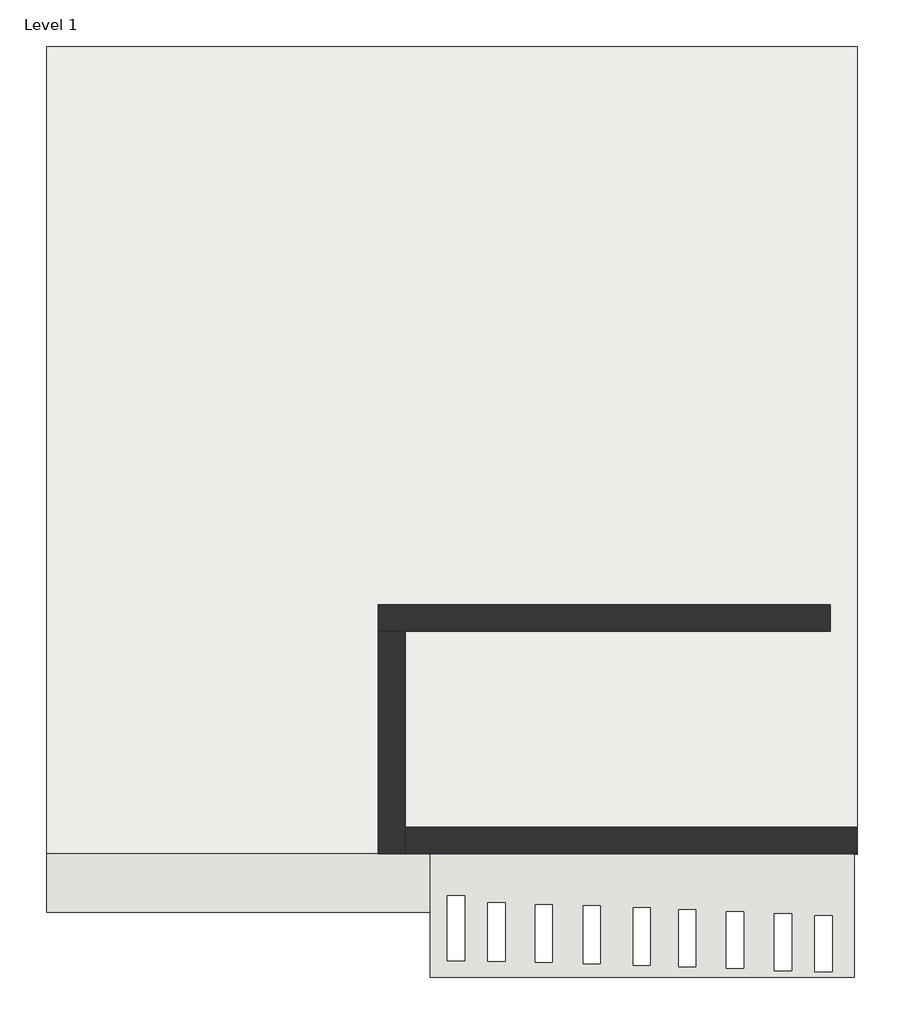
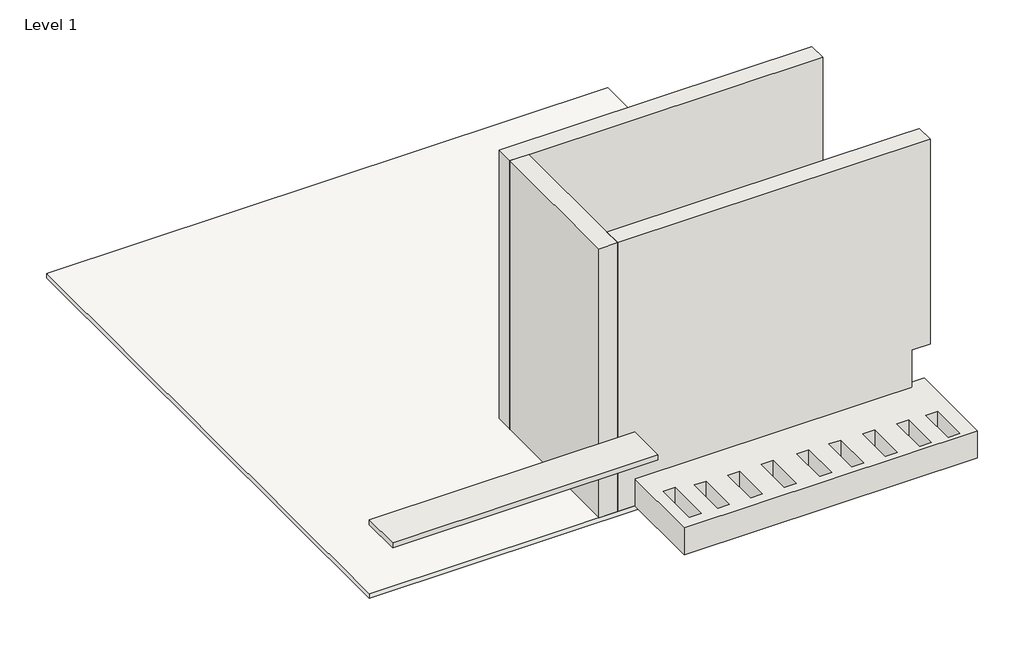
# One storey: 5 walls, 1 covering.
"""IFC4 building model written with IfcOpenShell, lengths in millimetres."""

from ifc_helpers import new_model, si_unit, frame, origin, place, context, project, spatial, polyline, outline, extrude, faceted_brep, transform, mapped, element, save
from components import walls_4_walls_4_fd780b34, walls_8_walls_8_172a5026

model = new_model("IFC4")

# Units and contexts
model_context = context("Model", 3, world=origin())
ifc_project = project(units=[si_unit("LENGTHUNIT", "METRE", prefix="MILLI")], contexts=[model_context])

# Site, building, storey
site = spatial("IfcSite", under=ifc_project)
building = spatial("IfcBuilding", under=site)
storey = spatial("IfcBuildingStorey", under=building, Name="Level 1", Elevation=3048.0)

# Covering
placement = place(None, origin())
element("IfcCovering", 1, ObjectType="600 x 1200mm grid", at=placement, inside=storey, context=model_context, shape_type="SweptSolid", body=[
    extrude(outline(polyline([(-15798.6897324, 2600.2819102), (-9784.4289001, 2600.2819102), (-9784.4289001, -3390.9180898), (-15798.6897324, -3390.9180898), (-15798.6897324, 2600.2819102)])), frame((0.0, 0.0, 2996.0), z_axis=(0.0, 0.0, 1.0), x_axis=(1.0, 0.0, 0.0)), (0.0, 0.0, 1.0), 52.0),
])

# Walls
element("IfcWall", 2, ObjectType="Generic - 9\"", at=placement, inside=storey, context=model_context, shape_type="Brep", body=[
    faceted_brep([(-9984.4289001, -3190.9180898, 3774.1343037), (-9984.4289001, -3190.9180898, 3048.0), (-13137.2289001, -3190.9180898, 3048.0), (-13137.2289001, -3190.9180898, 6096.0), (-9984.4289001, -3190.9180898, 6096.0), (-9784.4289001, -3190.9180898, 6096.0), (-9784.4289001, -3190.9180898, 3774.1343037), (-9984.4289001, -3390.9180898, 3048.0), (-9984.4289001, -3390.9180898, 3352.8), (-9984.4289001, -3390.9180898, 3774.1343037), (-9784.4289001, -3390.9180898, 3774.1343037), (-9784.4289001, -3390.9180898, 6096.0), (-13137.2289001, -3390.9180898, 6096.0), (-13137.2289001, -3390.9180898, 3048.0)], [[[0, 1, 2, 3, 4, 5, 6]], [[7, 8, 9, 10, 11, 12, 13]], [[2, 1, 7, 13]], [[5, 4, 3, 12, 11]], [[3, 2, 13, 12]], [[6, 10, 9, 0]], [[0, 9, 8, 7, 1]], [[6, 5, 11, 10]]]),
])
element("IfcWall", 3, ObjectType="Generic - 9\"", at=placement, inside=storey, context=model_context, shape_type="Brep", body=[
    faceted_brep([(-13337.2289001, -1739.9180898, 3048.0), (-13137.2289001, -1739.9180898, 3048.0), (-9984.4289001, -1739.9180898, 3048.0), (-9984.4289001, -1739.9180898, 6096.0), (-13137.2289001, -1739.9180898, 6096.0), (-13337.2289001, -1739.9180898, 6096.0), (-13337.2289001, -1539.9180898, 3048.0), (-13337.2289001, -1539.9180898, 6096.0), (-9984.4289001, -1539.9180898, 6096.0), (-9984.4289001, -1539.9180898, 3048.0)], [[[0, 1, 2, 3, 4, 5]], [[6, 7, 8, 9]], [[2, 1, 0, 6, 9]], [[5, 4, 3, 8, 7]], [[0, 5, 7, 6]], [[2, 9, 8, 3]]]),
])
element("IfcWall", 4, ObjectType="Generic - 9\"", at=placement, inside=storey, context=model_context, shape_type="Brep", body=[
    faceted_brep([(-13137.2289001, -3390.9180898, 3048.0), (-13137.2289001, -3190.9180898, 3048.0), (-13137.2289001, -1739.9180898, 3048.0), (-13137.2289001, -1739.9180898, 6096.0), (-13137.2289001, -3190.9180898, 6096.0), (-13137.2289001, -3390.9180898, 6096.0), (-13337.2289001, -3390.9180898, 3048.0), (-13337.2289001, -3390.9180898, 6096.0), (-13337.2289001, -1739.9180898, 6096.0), (-13337.2289001, -1739.9180898, 3048.0)], [[[0, 1, 2, 3, 4, 5]], [[6, 7, 8, 9]], [[2, 1, 0, 6, 9]], [[5, 4, 3, 8, 7]], [[0, 5, 7, 6]], [[3, 2, 9, 8]]]),
])
walls_4_walls_4_shape = walls_4_walls_4_fd780b34(model_context)
element("IfcWall", 5, ObjectType="Walls 4 : Walls 4", at=placement, inside=storey, context=model_context, shape_type="MappedRepresentation", body=[
    mapped(walls_4_walls_4_shape, transform((0.0, 0.0, 0.0), x_axis=(1.0, 0.0, 0.0), y_axis=(0.0, 1.0, 0.0), z_axis=(0.0, 0.0, 1.0))),
])
walls_8_walls_8_shape = walls_8_walls_8_172a5026(model_context)
element("IfcWall", 6, ObjectType="Walls 8 : Walls 8", at=placement, inside=storey, context=model_context, shape_type="MappedRepresentation", body=[
    mapped(walls_8_walls_8_shape, transform((0.0, 0.0, 0.0), x_axis=(1.0, 0.0, 0.0), y_axis=(0.0, 1.0, 0.0), z_axis=(0.0, 0.0, 1.0))),
])

save(model, "model.ifc")

# Revit data of these elements
# Type "600 x 1200mm grid"
#   built-in parameter 1002203 = 1 (stored number, unit not read)
#   built-in parameter 1002202 = 1 (stored number, unit not read)
#   Layers, outside or top first: 0' - 1.41732" "Default" (function 1); 0' - 0.62992" "Ceiling Tile 600 x 1200" (function 5)
# Type "Generic - 9\""
#   Layers, outside or top first: 0' - 7.87402" no material (function 1)
# Element 1 (IfcCovering, "600 x 1200mm grid")
#   Height Offset From Level = -0' - 2.04724"
#   Phase Created = New Construction
#   Materials on its faces: "Ceiling Tile 600 x 1200", "Default"
# Elements 2, 4 (IfcWall, "Generic - 9\"")
#   Top Offset = 0' - 0"
#   Base Offset = 0' - 0"
#   Unconnected Height = 10' - 0"
#   wall height = 10' - 0"
#   Phase Created = New Construction
#   Base Constraint = Level 1
#   Materials on its faces: "Default Wall", "Cherry"
# Element 3 (IfcWall, "Generic - 9\"")
#   Top Offset = 0' - 0"
#   Base Offset = 0' - 0"
#   Unconnected Height = 10' - 0"
#   wall height = 10' - 0"
#   Phase Created = New Construction
#   Base Constraint = Level 1
#   Materials on its faces: "Default Wall"
# Element 5 (IfcWall, "Walls 4 : Walls 4")
#   Phase Created = New Construction
#   Materials on its faces: "Default Wall"
# Element 6 (IfcWall, "Walls 8 : Walls 8")
#   Phase Created = New Construction
#   Materials on its faces: "Default Wall"
# Materials
#   "Default": colour RGB 80 80 80, transparency 0
#   "Ceiling Tile 600 x 1200": class "Generic", colour RGB 179 178 175, transparency 0, Description = "Acoustic ceiling tile", Cost = 0
#   "Default Wall": colour RGB 80 80 80, transparency 0
#   "Cherry": class "Wood", colour RGB 154 107 61, transparency 0, Description = "Prunus Serotina", Cost = 0
